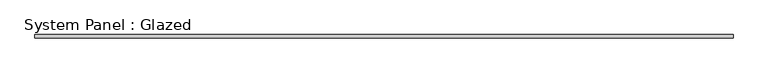
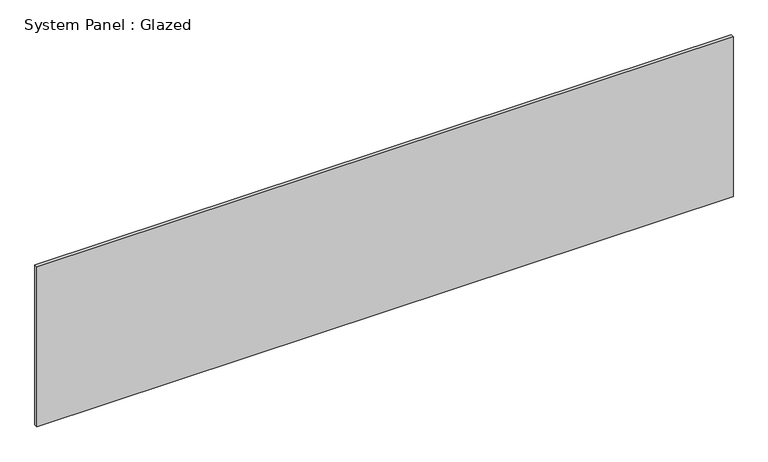
"""IFC4 building model written with IfcOpenShell, lengths in millimetres: plate geometry, System Panel : Glazed."""

from ifc_helpers import new_model, si_unit, origin, origin_with_axes, place, context, project, spatial, polyline, outline, extrude, source, transform, mapped, element, save


def system_panel_glazed_310057b8(model_context):
    return source(origin(), model_context, "Body", "SweptSolid", [
        extrude(outline(polyline([(2513.4709799, 19.05), (-2513.4709799, 19.05), (-2513.4709799, 44.45), (2513.4709799, 44.45), (2513.4709799, 19.05)])), origin_with_axes(), (0.0, 0.0, 1.0), 1219.2),
    ])


if __name__ == "__main__":
    model = new_model("IFC4")
    model_context = context("Model", 3, world=origin())
    ifc_project = project(units=[si_unit("LENGTHUNIT", "METRE", prefix="MILLI")], contexts=[model_context])
    site = spatial("IfcSite", under=ifc_project)
    building = spatial("IfcBuilding", under=site)
    placement = place(None, origin())
    system_panel_glazed_shape = system_panel_glazed_310057b8(model_context)
    element("IfcPlate", 1, ObjectType="System Panel : Glazed", at=placement, inside=building, context=model_context, shape_type="MappedRepresentation", body=[
        mapped(system_panel_glazed_shape, transform((0.0, 0.0, 0.0), x_axis=(1.0, 0.0, 0.0), y_axis=(0.0, 1.0, 0.0), z_axis=(0.0, 0.0, 1.0))),
    ])
    save(model, "model.ifc")

# Revit data of these elements
# Type "System Panel : Glazed"
#   Construction Type Id = "GSP4R"
#   Analytic Construction = "1/8 in Pilkington single glazing"
#   Visual Light Transmittance = 0.9
#   Solar Heat Gain Coefficient = 0.86
#   Heat Transfer Coefficient (U) = 1.18115 BTU/(h·ft²·°F)
# Element 1 (IfcPlate, "System Panel : Glazed")
#   Materials on its faces: "Glass"
# Materials
#   "Glass": class "Glass", colour RGB 0 128 192, transparency 0.75, Description = "Soda Lime Glass", Cost = 0
